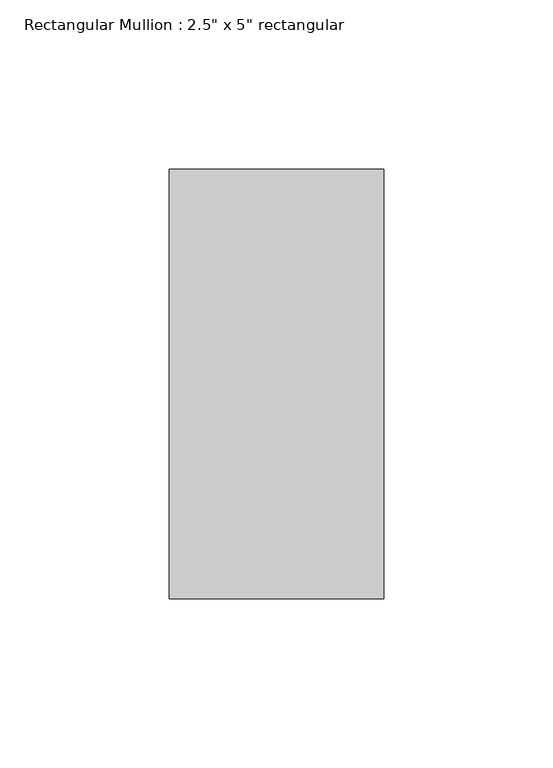
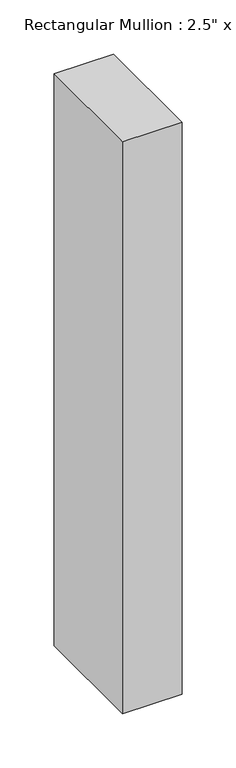
"""IFC4 building model written with IfcOpenShell, lengths in millimetres: member geometry."""

from ifc_helpers import new_model, si_unit, frame, origin, place, context, project, spatial, polyline, outline, extrude, source, transform, mapped, element, save


def member_61359a5b(model_context):
    return source(origin(), model_context, "Body", "SweptSolid", [
        extrude(outline(polyline([(0.0, 63.5), (0.0, -63.5), (-63.5, -63.5), (-63.5, 63.5), (0.0, 63.5)])), frame((0.0, 0.0, -645.5833333), z_axis=(0.0, 0.0, 1.0), x_axis=(1.0, 0.0, 0.0)), (0.0, 0.0, 1.0), 645.5833333),
    ])


if __name__ == "__main__":
    model = new_model("IFC4")
    model_context = context("Model", 3, world=origin())
    ifc_project = project(units=[si_unit("LENGTHUNIT", "METRE", prefix="MILLI")], contexts=[model_context])
    site = spatial("IfcSite", under=ifc_project)
    building = spatial("IfcBuilding", under=site)
    placement = place(None, origin())
    member_shape = member_61359a5b(model_context)
    element("IfcMember", 1, ObjectType="Rectangular Mullion : 2.5\" x 5\" rectangular", at=placement, inside=building, context=model_context, shape_type="MappedRepresentation", body=[
        mapped(member_shape, transform((0.0, 0.0, 0.0), x_axis=(1.0, 0.0, 0.0), y_axis=(0.0, 1.0, 0.0), z_axis=(0.0, 0.0, 1.0))),
    ])
    save(model, "model.ifc")

# Revit data of these elements
# Type "Rectangular Mullion : 2.5\" x 5\" rectangular"
#   built-in parameter 1007304 = 0.416667 (stored number, unit not read)
#   built-in parameter 1007301 = 0.104167 (stored number, unit not read)
#   built-in parameter 1007300 = 0.104167 (stored number, unit not read)
# Element 1 (IfcMember, "Rectangular Mullion : 2.5\" x 5\" rectangular")
#   Materials on its faces: "Aluminum"
# Materials
#   "Aluminum": class "Metal", colour RGB 247 247 247, transparency 0, Description = "Aluminum 6061", Cost = 0
